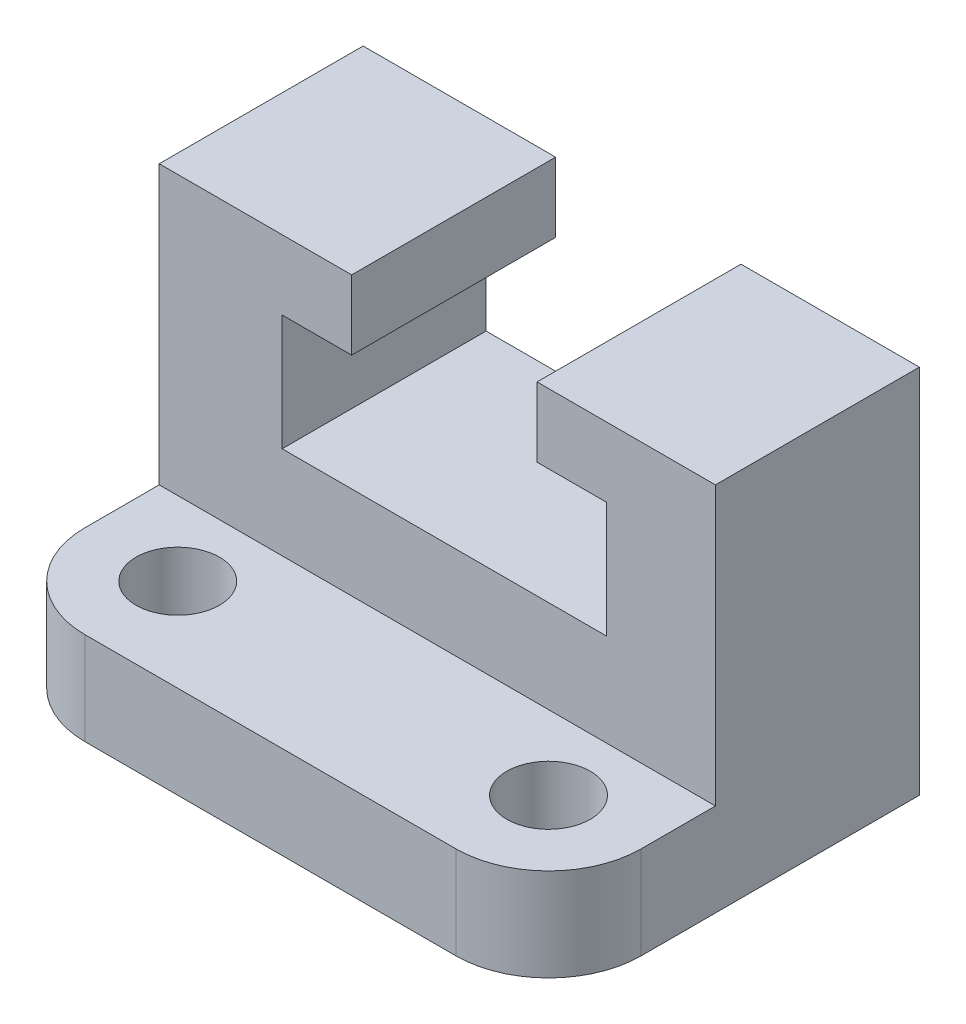
ISO-10303-21;
HEADER;
FILE_DESCRIPTION(('STEP AP214'),'2;1');
FILE_NAME('part.step','',(''),(''),'','','');
FILE_SCHEMA(('AUTOMOTIVE_DESIGN { 1 0 10303 214 1 1 1 1 }'));
ENDSEC;
DATA;
#1=APPLICATION_CONTEXT('core data for automotive mechanical design processes');
#2=APPLICATION_PROTOCOL_DEFINITION('international standard','automotive_design',2000,#1);
#3=PRODUCT_CONTEXT('',#1,'mechanical');
#4=PRODUCT('Part','Part','',(#3));
#5=PRODUCT_RELATED_PRODUCT_CATEGORY('part','',(#4));
#6=PRODUCT_DEFINITION_FORMATION('','',#4);
#7=PRODUCT_DEFINITION_CONTEXT('part definition',#1,'design');
#8=PRODUCT_DEFINITION('design','',#6,#7);
#9=PRODUCT_DEFINITION_SHAPE('','',#8);
#10=(LENGTH_UNIT() NAMED_UNIT(*) SI_UNIT(.MILLI.,.METRE.));
#11=(NAMED_UNIT(*) PLANE_ANGLE_UNIT() SI_UNIT($,.RADIAN.));
#12=(NAMED_UNIT(*) SI_UNIT($,.STERADIAN.) SOLID_ANGLE_UNIT());
#13=UNCERTAINTY_MEASURE_WITH_UNIT(LENGTH_MEASURE(1.E-05),#10,'distance_accuracy_value','');
#14=(GEOMETRIC_REPRESENTATION_CONTEXT(3) GLOBAL_UNCERTAINTY_ASSIGNED_CONTEXT((#13)) GLOBAL_UNIT_ASSIGNED_CONTEXT((#10,
#11,#12)) REPRESENTATION_CONTEXT('',''));
#15=CARTESIAN_POINT('',(0.,0.,0.));
#16=DIRECTION('',(0.,0.,1.));
#17=DIRECTION('',(1.,0.,0.));
#18=AXIS2_PLACEMENT_3D('',#15,#16,#17);
#19=CARTESIAN_POINT('',(0.,0.,22.));
#20=DIRECTION('',(0.,0.,1.));
#21=DIRECTION('',(1.,0.,0.));
#22=AXIS2_PLACEMENT_3D('',#19,#20,#21);
#23=PLANE('',#22);
#24=DIRECTION('',(0.,-1.,0.));
#25=VECTOR('',#24,1.);
#26=CARTESIAN_POINT('',(0.,40.,22.));
#27=LINE('',#26,#25);
#28=CARTESIAN_POINT('',(0.,40.,22.));
#29=VERTEX_POINT('',#28);
#30=CARTESIAN_POINT('',(0.,10.,22.));
#31=VERTEX_POINT('',#30);
#32=EDGE_CURVE('E61',#29,#31,#27,.T.);
#33=ORIENTED_EDGE('',*,*,#32,.T.);
#34=DIRECTION('',(1.,0.,0.));
#35=VECTOR('',#34,1.);
#36=CARTESIAN_POINT('',(0.,10.,22.));
#37=LINE('',#36,#35);
#38=CARTESIAN_POINT('',(60.,10.,22.));
#39=VERTEX_POINT('',#38);
#40=EDGE_CURVE('E57',#31,#39,#37,.T.);
#41=ORIENTED_EDGE('',*,*,#40,.T.);
#42=DIRECTION('',(0.,1.,0.));
#43=VECTOR('',#42,1.);
#44=CARTESIAN_POINT('',(60.,0.,22.));
#45=LINE('',#44,#43);
#46=CARTESIAN_POINT('',(60.,40.,22.));
#47=VERTEX_POINT('',#46);
#48=EDGE_CURVE('E200',#39,#47,#45,.T.);
#49=ORIENTED_EDGE('',*,*,#48,.T.);
#50=DIRECTION('',(-1.,0.,0.));
#51=VECTOR('',#50,1.);
#52=CARTESIAN_POINT('',(60.,40.,22.));
#53=LINE('',#52,#51);
#54=CARTESIAN_POINT('',(40.7619047619048,40.,22.));
#55=VERTEX_POINT('',#54);
#56=EDGE_CURVE('E205',#47,#55,#53,.T.);
#57=ORIENTED_EDGE('',*,*,#56,.T.);
#58=DIRECTION('',(0.,-1.,0.));
#59=VECTOR('',#58,1.);
#60=CARTESIAN_POINT('',(40.7619047619048,40.,22.));
#61=LINE('',#60,#59);
#62=CARTESIAN_POINT('',(40.7619047619048,32.5,22.));
#63=VERTEX_POINT('',#62);
#64=EDGE_CURVE('E204',#55,#63,#61,.T.);
#65=ORIENTED_EDGE('',*,*,#64,.T.);
#66=DIRECTION('',(1.,0.,0.));
#67=VECTOR('',#66,1.);
#68=CARTESIAN_POINT('',(40.7619047619048,32.5,22.));
#69=LINE('',#68,#67);
#70=CARTESIAN_POINT('',(48.2619047619048,32.5,22.));
#71=VERTEX_POINT('',#70);
#72=EDGE_CURVE('E206',#63,#71,#69,.T.);
#73=ORIENTED_EDGE('',*,*,#72,.T.);
#74=DIRECTION('',(0.,-1.,0.));
#75=VECTOR('',#74,1.);
#76=CARTESIAN_POINT('',(48.2619047619048,32.5,22.));
#77=LINE('',#76,#75);
#78=CARTESIAN_POINT('',(48.2619047619048,20.,22.));
#79=VERTEX_POINT('',#78);
#80=EDGE_CURVE('E208',#71,#79,#77,.T.);
#81=ORIENTED_EDGE('',*,*,#80,.T.);
#82=DIRECTION('',(-1.,0.,0.));
#83=VECTOR('',#82,1.);
#84=CARTESIAN_POINT('',(48.2619047619048,20.,22.));
#85=LINE('',#84,#83);
#86=CARTESIAN_POINT('',(13.2619047619048,20.,22.));
#87=VERTEX_POINT('',#86);
#88=EDGE_CURVE('E209',#79,#87,#85,.T.);
#89=ORIENTED_EDGE('',*,*,#88,.T.);
#90=DIRECTION('',(0.,1.,0.));
#91=VECTOR('',#90,1.);
#92=CARTESIAN_POINT('',(13.2619047619048,20.,22.));
#93=LINE('',#92,#91);
#94=CARTESIAN_POINT('',(13.2619047619048,32.5,22.));
#95=VERTEX_POINT('',#94);
#96=EDGE_CURVE('E215',#87,#95,#93,.T.);
#97=ORIENTED_EDGE('',*,*,#96,.T.);
#98=DIRECTION('',(1.,0.,0.));
#99=VECTOR('',#98,1.);
#100=CARTESIAN_POINT('',(13.2619047619048,32.5,22.));
#101=LINE('',#100,#99);
#102=CARTESIAN_POINT('',(20.7619047619048,32.5,22.));
#103=VERTEX_POINT('',#102);
#104=EDGE_CURVE('E212',#95,#103,#101,.T.);
#105=ORIENTED_EDGE('',*,*,#104,.T.);
#106=DIRECTION('',(0.,1.,0.));
#107=VECTOR('',#106,1.);
#108=CARTESIAN_POINT('',(20.7619047619048,32.5,22.));
#109=LINE('',#108,#107);
#110=CARTESIAN_POINT('',(20.7619047619048,40.,22.));
#111=VERTEX_POINT('',#110);
#112=EDGE_CURVE('E216',#103,#111,#109,.T.);
#113=ORIENTED_EDGE('',*,*,#112,.T.);
#114=DIRECTION('',(-1.,0.,0.));
#115=VECTOR('',#114,1.);
#116=CARTESIAN_POINT('',(20.7619047619048,40.,22.));
#117=LINE('',#116,#115);
#118=EDGE_CURVE('E217',#111,#29,#117,.T.);
#119=ORIENTED_EDGE('',*,*,#118,.T.);
#120=EDGE_LOOP('',(#33,#41,#49,#57,#65,#73,#81,#89,#97,#105,#113,#119));
#121=FACE_BOUND('',#120,.T.);
#122=ADVANCED_FACE('F41',(#121),#23,.T.);
#123=CARTESIAN_POINT('',(0.,40.,22.));
#124=DIRECTION('',(1.,0.,0.));
#125=DIRECTION('',(0.,1.,0.));
#126=AXIS2_PLACEMENT_3D('',#123,#124,#125);
#127=PLANE('',#126);
#128=DIRECTION('',(0.,0.,-1.));
#129=VECTOR('',#128,1.);
#130=CARTESIAN_POINT('',(0.,0.,22.));
#131=LINE('',#130,#129);
#132=CARTESIAN_POINT('',(0.,0.,29.9999999999999));
#133=VERTEX_POINT('',#132);
#134=CARTESIAN_POINT('',(0.,0.,0.));
#135=VERTEX_POINT('',#134);
#136=EDGE_CURVE('E11',#133,#135,#131,.T.);
#137=ORIENTED_EDGE('',*,*,#136,.F.);
#138=DIRECTION('',(0.,-1.,0.));
#139=VECTOR('',#138,1.);
#140=CARTESIAN_POINT('',(0.,10.,29.9999999999999));
#141=LINE('',#140,#139);
#142=CARTESIAN_POINT('',(0.,10.,29.9999999999999));
#143=VERTEX_POINT('',#142);
#144=EDGE_CURVE('E165',#143,#133,#141,.T.);
#145=ORIENTED_EDGE('',*,*,#144,.F.);
#146=DIRECTION('',(0.,0.,1.));
#147=VECTOR('',#146,1.);
#148=CARTESIAN_POINT('',(0.,10.,22.));
#149=LINE('',#148,#147);
#150=EDGE_CURVE('E155',#31,#143,#149,.T.);
#151=ORIENTED_EDGE('',*,*,#150,.F.);
#152=ORIENTED_EDGE('',*,*,#32,.F.);
#153=DIRECTION('',(0.,0.,-1.));
#154=VECTOR('',#153,1.);
#155=CARTESIAN_POINT('',(0.,40.,22.));
#156=LINE('',#155,#154);
#157=CARTESIAN_POINT('',(0.,40.,0.));
#158=VERTEX_POINT('',#157);
#159=EDGE_CURVE('E219',#29,#158,#156,.T.);
#160=ORIENTED_EDGE('',*,*,#159,.T.);
#161=DIRECTION('',(0.,-1.,0.));
#162=VECTOR('',#161,1.);
#163=CARTESIAN_POINT('',(0.,40.,0.));
#164=LINE('',#163,#162);
#165=EDGE_CURVE('E197',#158,#135,#164,.T.);
#166=ORIENTED_EDGE('',*,*,#165,.T.);
#167=EDGE_LOOP('',(#137,#145,#151,#152,#160,#166));
#168=FACE_BOUND('',#167,.T.);
#169=ADVANCED_FACE('F43',(#168),#127,.F.);
#170=CARTESIAN_POINT('',(0.,0.,22.));
#171=DIRECTION('',(0.,1.,0.));
#172=DIRECTION('',(0.,0.,1.));
#173=AXIS2_PLACEMENT_3D('',#170,#171,#172);
#174=PLANE('',#173);
#175=CARTESIAN_POINT('',(10.,0.,30.));
#176=DIRECTION('',(0.,1.,0.));
#177=DIRECTION('',(0.,0.,1.));
#178=AXIS2_PLACEMENT_3D('',#175,#176,#177);
#179=CIRCLE('',#178,4.5);
#180=CARTESIAN_POINT('',(10.,0.,34.5));
#181=VERTEX_POINT('',#180);
#182=EDGE_CURVE('E189',#181,#181,#179,.T.);
#183=ORIENTED_EDGE('',*,*,#182,.T.);
#184=EDGE_LOOP('',(#183));
#185=FACE_BOUND('',#184,.T.);
#186=CARTESIAN_POINT('',(50.,0.,30.));
#187=DIRECTION('',(0.,1.,0.));
#188=DIRECTION('',(0.,0.,1.));
#189=AXIS2_PLACEMENT_3D('',#186,#187,#188);
#190=CIRCLE('',#189,4.5);
#191=CARTESIAN_POINT('',(50.,0.,34.5));
#192=VERTEX_POINT('',#191);
#193=EDGE_CURVE('E179',#192,#192,#190,.T.);
#194=ORIENTED_EDGE('',*,*,#193,.T.);
#195=EDGE_LOOP('',(#194));
#196=FACE_BOUND('',#195,.T.);
#197=DIRECTION('',(1.,0.,0.));
#198=VECTOR('',#197,1.);
#199=CARTESIAN_POINT('',(0.,0.,0.));
#200=LINE('',#199,#198);
#201=CARTESIAN_POINT('',(60.,0.,0.));
#202=VERTEX_POINT('',#201);
#203=EDGE_CURVE('E225',#135,#202,#200,.T.);
#204=ORIENTED_EDGE('',*,*,#203,.T.);
#205=DIRECTION('',(0.,0.,-1.));
#206=VECTOR('',#205,1.);
#207=CARTESIAN_POINT('',(60.,0.,22.));
#208=LINE('',#207,#206);
#209=CARTESIAN_POINT('',(60.,0.,29.9999999999999));
#210=VERTEX_POINT('',#209);
#211=EDGE_CURVE('E47',#210,#202,#208,.T.);
#212=ORIENTED_EDGE('',*,*,#211,.F.);
#213=CARTESIAN_POINT('',(50.,0.,30.));
#214=DIRECTION('',(0.,-1.,0.));
#215=DIRECTION('',(0.,0.,-1.));
#216=AXIS2_PLACEMENT_3D('',#213,#214,#215);
#217=CIRCLE('',#216,10.);
#218=CARTESIAN_POINT('',(49.9999999999999,0.,40.));
#219=VERTEX_POINT('',#218);
#220=EDGE_CURVE('E175',#210,#219,#217,.T.);
#221=ORIENTED_EDGE('',*,*,#220,.T.);
#222=DIRECTION('',(1.,0.,0.));
#223=VECTOR('',#222,1.);
#224=CARTESIAN_POINT('',(10.0000000000001,0.,40.));
#225=LINE('',#224,#223);
#226=CARTESIAN_POINT('',(10.0000000000001,0.,40.));
#227=VERTEX_POINT('',#226);
#228=EDGE_CURVE('E172',#227,#219,#225,.T.);
#229=ORIENTED_EDGE('',*,*,#228,.F.);
#230=CARTESIAN_POINT('',(10.,0.,30.));
#231=DIRECTION('',(0.,-1.,0.));
#232=DIRECTION('',(0.,0.,-1.));
#233=AXIS2_PLACEMENT_3D('',#230,#231,#232);
#234=CIRCLE('',#233,10.);
#235=EDGE_CURVE('E186',#227,#133,#234,.T.);
#236=ORIENTED_EDGE('',*,*,#235,.T.);
#237=ORIENTED_EDGE('',*,*,#136,.T.);
#238=EDGE_LOOP('',(#204,#212,#221,#229,#236,#237));
#239=FACE_BOUND('',#238,.T.);
#240=ADVANCED_FACE('F301',(#185,#196,#239),#174,.F.);
#241=CARTESIAN_POINT('',(60.,0.,22.));
#242=DIRECTION('',(-1.,0.,0.));
#243=DIRECTION('',(0.,0.,1.));
#244=AXIS2_PLACEMENT_3D('',#241,#242,#243);
#245=PLANE('',#244);
#246=DIRECTION('',(0.,1.,0.));
#247=VECTOR('',#246,1.);
#248=CARTESIAN_POINT('',(60.,0.,0.));
#249=LINE('',#248,#247);
#250=CARTESIAN_POINT('',(60.,40.,0.));
#251=VERTEX_POINT('',#250);
#252=EDGE_CURVE('E221',#202,#251,#249,.T.);
#253=ORIENTED_EDGE('',*,*,#252,.T.);
#254=DIRECTION('',(0.,0.,-1.));
#255=VECTOR('',#254,1.);
#256=CARTESIAN_POINT('',(60.,40.,22.));
#257=LINE('',#256,#255);
#258=EDGE_CURVE('E267',#47,#251,#257,.T.);
#259=ORIENTED_EDGE('',*,*,#258,.F.);
#260=ORIENTED_EDGE('',*,*,#48,.F.);
#261=DIRECTION('',(0.,0.,1.));
#262=VECTOR('',#261,1.);
#263=CARTESIAN_POINT('',(60.,10.,0.));
#264=LINE('',#263,#262);
#265=CARTESIAN_POINT('',(60.,10.,29.9999999999999));
#266=VERTEX_POINT('',#265);
#267=EDGE_CURVE('E157',#39,#266,#264,.T.);
#268=ORIENTED_EDGE('',*,*,#267,.T.);
#269=DIRECTION('',(0.,-1.,0.));
#270=VECTOR('',#269,1.);
#271=CARTESIAN_POINT('',(60.,10.,29.9999999999999));
#272=LINE('',#271,#270);
#273=EDGE_CURVE('E167',#266,#210,#272,.T.);
#274=ORIENTED_EDGE('',*,*,#273,.T.);
#275=ORIENTED_EDGE('',*,*,#211,.T.);
#276=EDGE_LOOP('',(#253,#259,#260,#268,#274,#275));
#277=FACE_BOUND('',#276,.T.);
#278=ADVANCED_FACE('F273',(#277),#245,.F.);
#279=CARTESIAN_POINT('',(60.,40.,22.));
#280=DIRECTION('',(0.,-1.,0.));
#281=DIRECTION('',(0.,0.,-1.));
#282=AXIS2_PLACEMENT_3D('',#279,#280,#281);
#283=PLANE('',#282);
#284=DIRECTION('',(-1.,0.,0.));
#285=VECTOR('',#284,1.);
#286=CARTESIAN_POINT('',(60.,40.,0.));
#287=LINE('',#286,#285);
#288=CARTESIAN_POINT('',(40.7619047619048,40.,0.));
#289=VERTEX_POINT('',#288);
#290=EDGE_CURVE('E226',#251,#289,#287,.T.);
#291=ORIENTED_EDGE('',*,*,#290,.T.);
#292=DIRECTION('',(0.,0.,-1.));
#293=VECTOR('',#292,1.);
#294=CARTESIAN_POINT('',(40.7619047619048,40.,22.));
#295=LINE('',#294,#293);
#296=EDGE_CURVE('E266',#55,#289,#295,.T.);
#297=ORIENTED_EDGE('',*,*,#296,.F.);
#298=ORIENTED_EDGE('',*,*,#56,.F.);
#299=ORIENTED_EDGE('',*,*,#258,.T.);
#300=EDGE_LOOP('',(#291,#297,#298,#299));
#301=FACE_BOUND('',#300,.T.);
#302=ADVANCED_FACE('F289',(#301),#283,.F.);
#303=CARTESIAN_POINT('',(40.7619047619048,40.,22.));
#304=DIRECTION('',(1.,0.,0.));
#305=DIRECTION('',(0.,0.,-1.));
#306=AXIS2_PLACEMENT_3D('',#303,#304,#305);
#307=PLANE('',#306);
#308=DIRECTION('',(0.,-1.,0.));
#309=VECTOR('',#308,1.);
#310=CARTESIAN_POINT('',(40.7619047619048,40.,0.));
#311=LINE('',#310,#309);
#312=CARTESIAN_POINT('',(40.7619047619048,32.5,0.));
#313=VERTEX_POINT('',#312);
#314=EDGE_CURVE('E229',#289,#313,#311,.T.);
#315=ORIENTED_EDGE('',*,*,#314,.T.);
#316=DIRECTION('',(0.,0.,-1.));
#317=VECTOR('',#316,1.);
#318=CARTESIAN_POINT('',(40.7619047619048,32.5,22.));
#319=LINE('',#318,#317);
#320=EDGE_CURVE('E263',#63,#313,#319,.T.);
#321=ORIENTED_EDGE('',*,*,#320,.F.);
#322=ORIENTED_EDGE('',*,*,#64,.F.);
#323=ORIENTED_EDGE('',*,*,#296,.T.);
#324=EDGE_LOOP('',(#315,#321,#322,#323));
#325=FACE_BOUND('',#324,.T.);
#326=ADVANCED_FACE('F295',(#325),#307,.F.);
#327=CARTESIAN_POINT('',(40.7619047619048,32.5,22.));
#328=DIRECTION('',(0.,1.,0.));
#329=DIRECTION('',(0.,0.,1.));
#330=AXIS2_PLACEMENT_3D('',#327,#328,#329);
#331=PLANE('',#330);
#332=DIRECTION('',(1.,0.,0.));
#333=VECTOR('',#332,1.);
#334=CARTESIAN_POINT('',(40.7619047619048,32.5,0.));
#335=LINE('',#334,#333);
#336=CARTESIAN_POINT('',(48.2619047619048,32.5,0.));
#337=VERTEX_POINT('',#336);
#338=EDGE_CURVE('E230',#313,#337,#335,.T.);
#339=ORIENTED_EDGE('',*,*,#338,.T.);
#340=DIRECTION('',(0.,0.,-1.));
#341=VECTOR('',#340,1.);
#342=CARTESIAN_POINT('',(48.2619047619048,32.5,22.));
#343=LINE('',#342,#341);
#344=EDGE_CURVE('E257',#71,#337,#343,.T.);
#345=ORIENTED_EDGE('',*,*,#344,.F.);
#346=ORIENTED_EDGE('',*,*,#72,.F.);
#347=ORIENTED_EDGE('',*,*,#320,.T.);
#348=EDGE_LOOP('',(#339,#345,#346,#347));
#349=FACE_BOUND('',#348,.T.);
#350=ADVANCED_FACE('F343',(#349),#331,.F.);
#351=CARTESIAN_POINT('',(48.2619047619048,32.5,22.));
#352=DIRECTION('',(1.,0.,0.));
#353=DIRECTION('',(0.,0.,-1.));
#354=AXIS2_PLACEMENT_3D('',#351,#352,#353);
#355=PLANE('',#354);
#356=DIRECTION('',(0.,-1.,0.));
#357=VECTOR('',#356,1.);
#358=CARTESIAN_POINT('',(48.2619047619048,32.5,0.));
#359=LINE('',#358,#357);
#360=CARTESIAN_POINT('',(48.2619047619048,20.,0.));
#361=VERTEX_POINT('',#360);
#362=EDGE_CURVE('E232',#337,#361,#359,.T.);
#363=ORIENTED_EDGE('',*,*,#362,.T.);
#364=DIRECTION('',(0.,0.,-1.));
#365=VECTOR('',#364,1.);
#366=CARTESIAN_POINT('',(48.2619047619048,20.,22.));
#367=LINE('',#366,#365);
#368=EDGE_CURVE('E260',#79,#361,#367,.T.);
#369=ORIENTED_EDGE('',*,*,#368,.F.);
#370=ORIENTED_EDGE('',*,*,#80,.F.);
#371=ORIENTED_EDGE('',*,*,#344,.T.);
#372=EDGE_LOOP('',(#363,#369,#370,#371));
#373=FACE_BOUND('',#372,.T.);
#374=ADVANCED_FACE('F340',(#373),#355,.F.);
#375=CARTESIAN_POINT('',(48.2619047619048,20.,22.));
#376=DIRECTION('',(0.,-1.,0.));
#377=DIRECTION('',(1.,0.,0.));
#378=AXIS2_PLACEMENT_3D('',#375,#376,#377);
#379=PLANE('',#378);
#380=DIRECTION('',(-1.,0.,0.));
#381=VECTOR('',#380,1.);
#382=CARTESIAN_POINT('',(48.2619047619048,20.,0.));
#383=LINE('',#382,#381);
#384=CARTESIAN_POINT('',(13.2619047619048,20.,0.));
#385=VERTEX_POINT('',#384);
#386=EDGE_CURVE('E233',#361,#385,#383,.T.);
#387=ORIENTED_EDGE('',*,*,#386,.T.);
#388=DIRECTION('',(0.,0.,-1.));
#389=VECTOR('',#388,1.);
#390=CARTESIAN_POINT('',(13.2619047619048,20.,22.));
#391=LINE('',#390,#389);
#392=EDGE_CURVE('E255',#87,#385,#391,.T.);
#393=ORIENTED_EDGE('',*,*,#392,.F.);
#394=ORIENTED_EDGE('',*,*,#88,.F.);
#395=ORIENTED_EDGE('',*,*,#368,.T.);
#396=EDGE_LOOP('',(#387,#393,#394,#395));
#397=FACE_BOUND('',#396,.T.);
#398=ADVANCED_FACE('F336',(#397),#379,.F.);
#399=CARTESIAN_POINT('',(13.2619047619048,20.,22.));
#400=DIRECTION('',(-1.,0.,0.));
#401=DIRECTION('',(0.,0.,1.));
#402=AXIS2_PLACEMENT_3D('',#399,#400,#401);
#403=PLANE('',#402);
#404=DIRECTION('',(0.,1.,0.));
#405=VECTOR('',#404,1.);
#406=CARTESIAN_POINT('',(13.2619047619048,20.,0.));
#407=LINE('',#406,#405);
#408=CARTESIAN_POINT('',(13.2619047619048,32.5,0.));
#409=VERTEX_POINT('',#408);
#410=EDGE_CURVE('E237',#385,#409,#407,.T.);
#411=ORIENTED_EDGE('',*,*,#410,.T.);
#412=DIRECTION('',(0.,0.,-1.));
#413=VECTOR('',#412,1.);
#414=CARTESIAN_POINT('',(13.2619047619048,32.5,22.));
#415=LINE('',#414,#413);
#416=EDGE_CURVE('E253',#95,#409,#415,.T.);
#417=ORIENTED_EDGE('',*,*,#416,.F.);
#418=ORIENTED_EDGE('',*,*,#96,.F.);
#419=ORIENTED_EDGE('',*,*,#392,.T.);
#420=EDGE_LOOP('',(#411,#417,#418,#419));
#421=FACE_BOUND('',#420,.T.);
#422=ADVANCED_FACE('F335',(#421),#403,.F.);
#423=CARTESIAN_POINT('',(13.2619047619048,32.5,22.));
#424=DIRECTION('',(0.,1.,0.));
#425=DIRECTION('',(0.,0.,1.));
#426=AXIS2_PLACEMENT_3D('',#423,#424,#425);
#427=PLANE('',#426);
#428=DIRECTION('',(1.,0.,0.));
#429=VECTOR('',#428,1.);
#430=CARTESIAN_POINT('',(13.2619047619048,32.5,0.));
#431=LINE('',#430,#429);
#432=CARTESIAN_POINT('',(20.7619047619048,32.5,0.));
#433=VERTEX_POINT('',#432);
#434=EDGE_CURVE('E236',#409,#433,#431,.T.);
#435=ORIENTED_EDGE('',*,*,#434,.T.);
#436=DIRECTION('',(0.,0.,-1.));
#437=VECTOR('',#436,1.);
#438=CARTESIAN_POINT('',(20.7619047619048,32.5,22.));
#439=LINE('',#438,#437);
#440=EDGE_CURVE('E249',#103,#433,#439,.T.);
#441=ORIENTED_EDGE('',*,*,#440,.F.);
#442=ORIENTED_EDGE('',*,*,#104,.F.);
#443=ORIENTED_EDGE('',*,*,#416,.T.);
#444=EDGE_LOOP('',(#435,#441,#442,#443));
#445=FACE_BOUND('',#444,.T.);
#446=ADVANCED_FACE('F327',(#445),#427,.F.);
#447=CARTESIAN_POINT('',(20.7619047619048,32.5,22.));
#448=DIRECTION('',(-1.,0.,0.));
#449=DIRECTION('',(0.,-1.,0.));
#450=AXIS2_PLACEMENT_3D('',#447,#448,#449);
#451=PLANE('',#450);
#452=DIRECTION('',(0.,1.,0.));
#453=VECTOR('',#452,1.);
#454=CARTESIAN_POINT('',(20.7619047619048,32.5,0.));
#455=LINE('',#454,#453);
#456=CARTESIAN_POINT('',(20.7619047619048,40.,0.));
#457=VERTEX_POINT('',#456);
#458=EDGE_CURVE('E238',#433,#457,#455,.T.);
#459=ORIENTED_EDGE('',*,*,#458,.T.);
#460=DIRECTION('',(0.,0.,-1.));
#461=VECTOR('',#460,1.);
#462=CARTESIAN_POINT('',(20.7619047619048,40.,22.));
#463=LINE('',#462,#461);
#464=EDGE_CURVE('E245',#111,#457,#463,.T.);
#465=ORIENTED_EDGE('',*,*,#464,.F.);
#466=ORIENTED_EDGE('',*,*,#112,.F.);
#467=ORIENTED_EDGE('',*,*,#440,.T.);
#468=EDGE_LOOP('',(#459,#465,#466,#467));
#469=FACE_BOUND('',#468,.T.);
#470=ADVANCED_FACE('F322',(#469),#451,.F.);
#471=CARTESIAN_POINT('',(20.7619047619048,40.,22.));
#472=DIRECTION('',(0.,-1.,0.));
#473=DIRECTION('',(0.,0.,-1.));
#474=AXIS2_PLACEMENT_3D('',#471,#472,#473);
#475=PLANE('',#474);
#476=DIRECTION('',(-1.,0.,0.));
#477=VECTOR('',#476,1.);
#478=CARTESIAN_POINT('',(20.7619047619048,40.,0.));
#479=LINE('',#478,#477);
#480=EDGE_CURVE('E199',#457,#158,#479,.T.);
#481=ORIENTED_EDGE('',*,*,#480,.T.);
#482=ORIENTED_EDGE('',*,*,#159,.F.);
#483=ORIENTED_EDGE('',*,*,#118,.F.);
#484=ORIENTED_EDGE('',*,*,#464,.T.);
#485=EDGE_LOOP('',(#481,#482,#483,#484));
#486=FACE_BOUND('',#485,.T.);
#487=ADVANCED_FACE('F325',(#486),#475,.F.);
#488=CARTESIAN_POINT('',(0.,0.,0.));
#489=DIRECTION('',(0.,0.,1.));
#490=DIRECTION('',(1.,0.,0.));
#491=AXIS2_PLACEMENT_3D('',#488,#489,#490);
#492=PLANE('',#491);
#493=ORIENTED_EDGE('',*,*,#203,.F.);
#494=ORIENTED_EDGE('',*,*,#165,.F.);
#495=ORIENTED_EDGE('',*,*,#480,.F.);
#496=ORIENTED_EDGE('',*,*,#458,.F.);
#497=ORIENTED_EDGE('',*,*,#434,.F.);
#498=ORIENTED_EDGE('',*,*,#410,.F.);
#499=ORIENTED_EDGE('',*,*,#386,.F.);
#500=ORIENTED_EDGE('',*,*,#362,.F.);
#501=ORIENTED_EDGE('',*,*,#338,.F.);
#502=ORIENTED_EDGE('',*,*,#314,.F.);
#503=ORIENTED_EDGE('',*,*,#290,.F.);
#504=ORIENTED_EDGE('',*,*,#252,.F.);
#505=EDGE_LOOP('',(#493,#494,#495,#496,#497,#498,#499,#500,#501,#502,#503,#504));
#506=FACE_BOUND('',#505,.T.);
#507=ADVANCED_FACE('F282',(#506),#492,.F.);
#508=CARTESIAN_POINT('',(10.,10.,30.));
#509=DIRECTION('',(0.,-1.,0.));
#510=DIRECTION('',(0.,0.,-1.));
#511=AXIS2_PLACEMENT_3D('',#508,#509,#510);
#512=CYLINDRICAL_SURFACE('',#511,10.);
#513=ORIENTED_EDGE('',*,*,#235,.F.);
#514=DIRECTION('',(0.,-1.,0.));
#515=VECTOR('',#514,1.);
#516=CARTESIAN_POINT('',(10.0000000000001,10.,40.));
#517=LINE('',#516,#515);
#518=CARTESIAN_POINT('',(10.0000000000001,10.,40.));
#519=VERTEX_POINT('',#518);
#520=EDGE_CURVE('E168',#519,#227,#517,.T.);
#521=ORIENTED_EDGE('',*,*,#520,.F.);
#522=CARTESIAN_POINT('',(10.,10.,30.));
#523=DIRECTION('',(0.,-1.,0.));
#524=DIRECTION('',(0.,0.,-1.));
#525=AXIS2_PLACEMENT_3D('',#522,#523,#524);
#526=CIRCLE('',#525,10.);
#527=EDGE_CURVE('E156',#519,#143,#526,.T.);
#528=ORIENTED_EDGE('',*,*,#527,.T.);
#529=ORIENTED_EDGE('',*,*,#144,.T.);
#530=EDGE_LOOP('',(#513,#521,#528,#529));
#531=FACE_BOUND('',#530,.T.);
#532=ADVANCED_FACE('F166',(#531),#512,.T.);
#533=CARTESIAN_POINT('',(10.0000000000001,10.,40.));
#534=DIRECTION('',(0.,0.,-1.));
#535=DIRECTION('',(-1.,0.,0.));
#536=AXIS2_PLACEMENT_3D('',#533,#534,#535);
#537=PLANE('',#536);
#538=ORIENTED_EDGE('',*,*,#228,.T.);
#539=DIRECTION('',(0.,-1.,0.));
#540=VECTOR('',#539,1.);
#541=CARTESIAN_POINT('',(49.9999999999999,10.,40.));
#542=LINE('',#541,#540);
#543=CARTESIAN_POINT('',(49.9999999999999,10.,40.));
#544=VERTEX_POINT('',#543);
#545=EDGE_CURVE('E192',#544,#219,#542,.T.);
#546=ORIENTED_EDGE('',*,*,#545,.F.);
#547=DIRECTION('',(1.,0.,0.));
#548=VECTOR('',#547,1.);
#549=CARTESIAN_POINT('',(10.0000000000001,10.,40.));
#550=LINE('',#549,#548);
#551=EDGE_CURVE('E170',#519,#544,#550,.T.);
#552=ORIENTED_EDGE('',*,*,#551,.F.);
#553=ORIENTED_EDGE('',*,*,#520,.T.);
#554=EDGE_LOOP('',(#538,#546,#552,#553));
#555=FACE_BOUND('',#554,.T.);
#556=ADVANCED_FACE('F304',(#555),#537,.F.);
#557=CARTESIAN_POINT('',(50.,10.,30.));
#558=DIRECTION('',(0.,-1.,0.));
#559=DIRECTION('',(0.,0.,-1.));
#560=AXIS2_PLACEMENT_3D('',#557,#558,#559);
#561=CYLINDRICAL_SURFACE('',#560,10.);
#562=ORIENTED_EDGE('',*,*,#220,.F.);
#563=ORIENTED_EDGE('',*,*,#273,.F.);
#564=CARTESIAN_POINT('',(50.,10.,30.));
#565=DIRECTION('',(0.,-1.,0.));
#566=DIRECTION('',(0.,0.,-1.));
#567=AXIS2_PLACEMENT_3D('',#564,#565,#566);
#568=CIRCLE('',#567,10.);
#569=EDGE_CURVE('E185',#266,#544,#568,.T.);
#570=ORIENTED_EDGE('',*,*,#569,.T.);
#571=ORIENTED_EDGE('',*,*,#545,.T.);
#572=EDGE_LOOP('',(#562,#563,#570,#571));
#573=FACE_BOUND('',#572,.T.);
#574=ADVANCED_FACE('F298',(#573),#561,.T.);
#575=CARTESIAN_POINT('',(10.,10.,30.));
#576=DIRECTION('',(0.,-1.,0.));
#577=DIRECTION('',(0.,0.,-1.));
#578=AXIS2_PLACEMENT_3D('',#575,#576,#577);
#579=PLANE('',#578);
#580=CARTESIAN_POINT('',(10.,10.,30.));
#581=DIRECTION('',(0.,1.,0.));
#582=DIRECTION('',(0.,0.,1.));
#583=AXIS2_PLACEMENT_3D('',#580,#581,#582);
#584=CIRCLE('',#583,4.5);
#585=CARTESIAN_POINT('',(10.,10.,34.5));
#586=VERTEX_POINT('',#585);
#587=EDGE_CURVE('E370',#586,#586,#584,.T.);
#588=ORIENTED_EDGE('',*,*,#587,.F.);
#589=EDGE_LOOP('',(#588));
#590=FACE_BOUND('',#589,.T.);
#591=CARTESIAN_POINT('',(50.,10.,30.));
#592=DIRECTION('',(0.,1.,0.));
#593=DIRECTION('',(0.,0.,1.));
#594=AXIS2_PLACEMENT_3D('',#591,#592,#593);
#595=CIRCLE('',#594,4.5);
#596=CARTESIAN_POINT('',(50.,10.,34.5));
#597=VERTEX_POINT('',#596);
#598=EDGE_CURVE('E364',#597,#597,#595,.T.);
#599=ORIENTED_EDGE('',*,*,#598,.F.);
#600=EDGE_LOOP('',(#599));
#601=FACE_BOUND('',#600,.T.);
#602=ORIENTED_EDGE('',*,*,#40,.F.);
#603=ORIENTED_EDGE('',*,*,#150,.T.);
#604=ORIENTED_EDGE('',*,*,#527,.F.);
#605=ORIENTED_EDGE('',*,*,#551,.T.);
#606=ORIENTED_EDGE('',*,*,#569,.F.);
#607=ORIENTED_EDGE('',*,*,#267,.F.);
#608=EDGE_LOOP('',(#602,#603,#604,#605,#606,#607));
#609=FACE_BOUND('',#608,.T.);
#610=ADVANCED_FACE('F152',(#590,#601,#609),#579,.F.);
#611=CARTESIAN_POINT('',(50.,0.,30.));
#612=DIRECTION('',(0.,1.,0.));
#613=DIRECTION('',(0.,0.,1.));
#614=AXIS2_PLACEMENT_3D('',#611,#612,#613);
#615=CYLINDRICAL_SURFACE('',#614,4.5);
#616=ORIENTED_EDGE('',*,*,#193,.F.);
#617=EDGE_LOOP('',(#616));
#618=FACE_BOUND('',#617,.T.);
#619=ORIENTED_EDGE('',*,*,#598,.T.);
#620=EDGE_LOOP('',(#619));
#621=FACE_BOUND('',#620,.T.);
#622=ADVANCED_FACE('F378',(#618,#621),#615,.F.);
#623=CARTESIAN_POINT('',(10.,0.,30.));
#624=DIRECTION('',(0.,1.,0.));
#625=DIRECTION('',(0.,0.,1.));
#626=AXIS2_PLACEMENT_3D('',#623,#624,#625);
#627=CYLINDRICAL_SURFACE('',#626,4.5);
#628=ORIENTED_EDGE('',*,*,#182,.F.);
#629=EDGE_LOOP('',(#628));
#630=FACE_BOUND('',#629,.T.);
#631=ORIENTED_EDGE('',*,*,#587,.T.);
#632=EDGE_LOOP('',(#631));
#633=FACE_BOUND('',#632,.T.);
#634=ADVANCED_FACE('F374',(#630,#633),#627,.F.);
#635=CLOSED_SHELL('',(#122,#169,#240,#278,#302,#326,#350,#374,#398,#422,#446,#470,#487,#507,
#532,#556,#574,#610,#622,#634));
#636=MANIFOLD_SOLID_BREP('B2',#635);
#637=ADVANCED_BREP_SHAPE_REPRESENTATION('',(#18,#636),#14);
#638=SHAPE_DEFINITION_REPRESENTATION(#9,#637);
ENDSEC;
END-ISO-10303-21;
